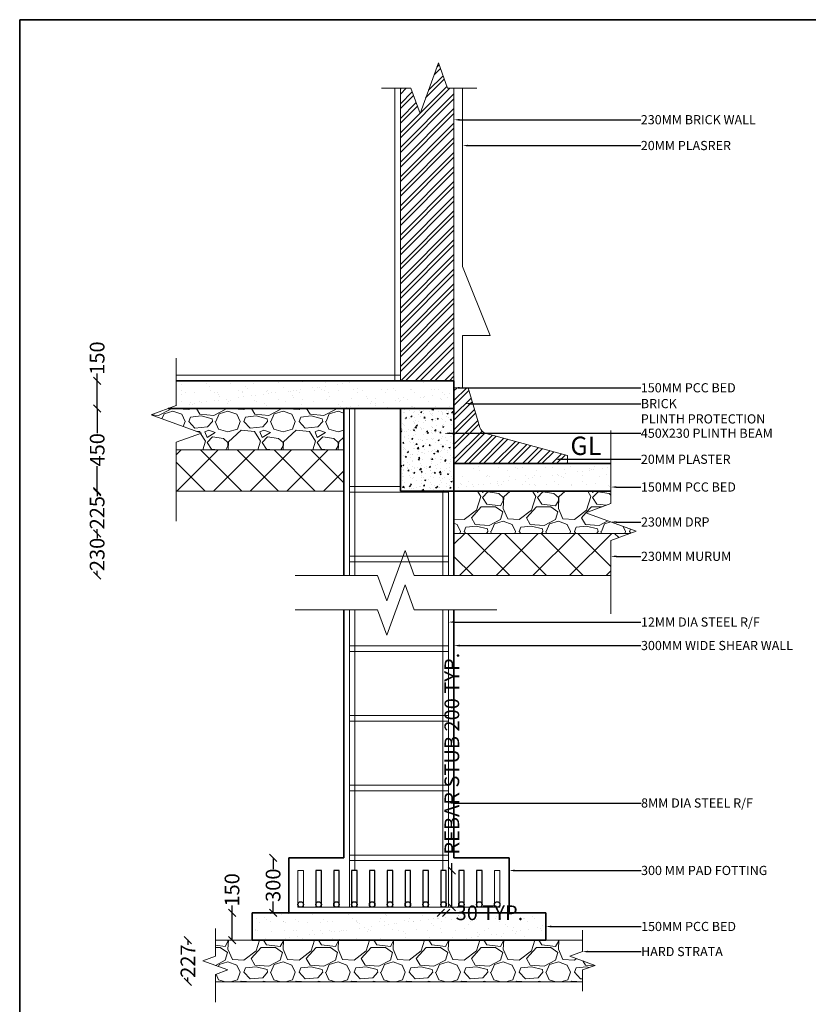
# Model space of a CAD drawing. Units: millimetres. Extents: x -6233 to 6805, y -5269 to 4890.
# Tile 2 of 4: x -6233 to -1936, y -472 to 4890. Entities that reach past the tile are written whole.
import ezdxf
from ezdxf import colors
from ezdxf.entities.mleader import LeaderData, LeaderLine
from ezdxf.math import Vec2, Vec3

# ---------------------------------------------------------------- set-up
doc = ezdxf.new("R2010")
doc.units = ezdxf.units.MM
doc.header["$MEASUREMENT"] = 0
for name, color, linetype, lineweight in [('S-ANNO-DIMS', 2, 'Continuous', 18), ('S-ANNO-TEXT', 3, 'Continuous', 18), ('S-ANNO-TTLB', 7, 'Continuous', 35), ('S-CONC', 7, 'Continuous', 35), ('S-FNDN', 8, 'Continuous', 18), ('S-PATT', 252, 'Continuous', 13), ('S-REIN', 1, 'Continuous', 25)]:
    doc.layers.add(name, color=color, linetype=linetype, lineweight=lineweight)
doc.styles.get("Standard").update_dxf_attribs({"font": 'arial.ttf'})
doc.dimstyles.get("Standard").update_dxf_attribs({"dimtxt": 80, "dimasz": 40, "dimexe": 0.18, "dimexo": 0.0625, "dimgap": 0.09, "dimtad": 0, "dimdec": 0, "dimzin": 0, "dimdsep": 46, "dimtxsty": 'Standard', "dimblk": 'OBLIQUE', "dimcen": 0.09, "dimadec": 0, "dimazin": 0, "dimtfac": 1, "dimtdec": 0, "dimtofl": 0, "dimtmove": 0, "dimatfit": 3, "dimfxl": 1, "dimfxlon": 1, "dimtolj": 1, "dimtzin": 0, "dimarcsym": 0})

# ---------------------------------------------------------------- blocks, each defined once
blk = doc.blocks.new('_Oblique')
at = {"color": 0, "linetype": 'ByBlock', "lineweight": -2}
blk.add_line((-0.5, -0.5), (0.5, 0.5), dxfattribs=at)
blk = doc.blocks.new('*D2')
at = {"layer": 'DEFPOINTS', "color": 0, "transparency": 16777216}
for p in [(-5316.4, -123.9), (-5166.8, -123.9), (-5166.8, -350.9)]:
    blk.add_point(p, dxfattribs=at)
at = {"layer": 'S-ANNO-DIMS', "color": 0, "lineweight": -2, "transparency": 16777216}
for p, q in [((-5315.4, -123.9), (-5316.6, -123.9)), ((-5316.4, -123.9), (-5316.4, -148.2)), ((-5315.4, -350.9), (-5316.6, -350.9)), ((-5316.4, -350.9), (-5316.4, -326.5))]:
    blk.add_line(p, q, dxfattribs=at)
at = {"layer": 'S-ANNO-DIMS', "color": 0, "lineweight": -2, "transparency": 16777216, "xscale": 40, "yscale": 40, "zscale": 40}
for p, rotation in [((-5316.4, -123.9), 90), ((-5316.4, -350.9), 270)]:
    blk.add_blockref('_Oblique', p, dxfattribs=dict(at, rotation=rotation))
at = {"layer": 'S-ANNO-DIMS', "color": 0, "transparency": 16777216, "insert": (-5316.4, -237.4), "char_height": 80, "attachment_point": 5, "rotation": 90}
blk.add_mtext('\\A1;227', dxfattribs=at)
blk = doc.blocks.new('*D3')
at = {"layer": 'DEFPOINTS', "color": 0, "transparency": 16777216}
for p in [(-5076.2, 26.1), (-4966.8, 26.1), (-4966.8, -123.9)]:
    blk.add_point(p, dxfattribs=at)
at = {"layer": 'S-ANNO-DIMS', "color": 0, "lineweight": -2, "transparency": 16777216}
for p, q in [((-5076.2, 26.1), (-5076.2, 66.1)), ((-5075.2, 26.1), (-5076.4, 26.1)), ((-5076.2, -123.9), (-5076.2, 26.1)), ((-5075.2, -123.9), (-5076.4, -123.9))]:
    blk.add_line(p, q, dxfattribs=at)
at = {"layer": 'S-ANNO-DIMS', "color": 0, "lineweight": -2, "transparency": 16777216, "xscale": 40, "yscale": 40, "zscale": 40}
for p, rotation in [((-5076.2, 26.1), 90), ((-5076.2, -123.9), 270)]:
    blk.add_blockref('_Oblique', p, dxfattribs=dict(at, rotation=rotation))
at = {"layer": 'S-ANNO-DIMS', "color": 0, "transparency": 16777216, "insert": (-5076.2, 150.7), "char_height": 80, "attachment_point": 5, "rotation": 90}
blk.add_mtext('\\A1;150', dxfattribs=at)
blk = doc.blocks.new('*D4')
at = {"layer": 'DEFPOINTS', "color": 0, "transparency": 16777216}
for p in [(-4852.4, 326.1), (-4766.8, 326.1), (-4766.8, 26.1)]:
    blk.add_point(p, dxfattribs=at)
at = {"layer": 'S-ANNO-DIMS', "color": 0, "lineweight": -2, "transparency": 16777216}
for p, q in [((-4851.4, 326.1), (-4852.6, 326.1)), ((-4852.4, 326.1), (-4852.4, 264.4)), ((-4852.4, 26.1), (-4852.4, 87.8)), ((-4851.4, 26.1), (-4852.6, 26.1))]:
    blk.add_line(p, q, dxfattribs=at)
at = {"layer": 'S-ANNO-DIMS', "color": 0, "lineweight": -2, "transparency": 16777216, "xscale": 40, "yscale": 40, "zscale": 40}
for p, rotation in [((-4852.4, 326.1), 90), ((-4852.4, 26.1), 270)]:
    blk.add_blockref('_Oblique', p, dxfattribs=dict(at, rotation=rotation))
at = {"layer": 'S-ANNO-DIMS', "color": 0, "transparency": 16777216, "insert": (-4852.4, 176.1), "char_height": 80, "attachment_point": 5, "rotation": 90}
blk.add_mtext('\\A1;300', dxfattribs=at)
blk = doc.blocks.new('*D5')
at = {"layer": 'DEFPOINTS', "color": 0, "transparency": 16777216}
for p in [(-5810.9, 2092.6), (-3866.8, 2092.6), (-3858.6, 1862.6)]:
    blk.add_point(p, dxfattribs=at)
at = {"layer": 'S-ANNO-DIMS', "color": 0, "lineweight": -2, "transparency": 16777216}
for p, q in [((-5809.9, 2092.6), (-5811.1, 2092.6)), ((-5810.9, 2092.6), (-5810.9, 2066.7)), ((-5810.9, 1862.6), (-5810.9, 1888.6)), ((-5809.9, 1862.6), (-5811.1, 1862.6))]:
    blk.add_line(p, q, dxfattribs=at)
at = {"layer": 'S-ANNO-DIMS', "color": 0, "lineweight": -2, "transparency": 16777216, "xscale": 40, "yscale": 40, "zscale": 40}
for p, rotation in [((-5810.9, 2092.6), 90), ((-5810.9, 1862.6), 270)]:
    blk.add_blockref('_Oblique', p, dxfattribs=dict(at, rotation=rotation))
at = {"layer": 'S-ANNO-DIMS', "color": 0, "transparency": 16777216, "insert": (-5810.9, 1977.6), "char_height": 80, "attachment_point": 5, "rotation": 90}
blk.add_mtext('\\A1;230', dxfattribs=at)
blk = doc.blocks.new('*D6')
at = {"layer": 'DEFPOINTS', "color": 0, "transparency": 16777216}
for p in [(-5811.1, 2317.5), (-3866.8, 2317.5), (-3866.8, 2092.6)]:
    blk.add_point(p, dxfattribs=at)
at = {"layer": 'S-ANNO-DIMS', "color": 0, "lineweight": -2, "transparency": 16777216}
for p, q in [((-5810.1, 2317.5), (-5811.3, 2317.5)), ((-5811.1, 2317.5), (-5811.1, 2294.5)), ((-5810.1, 2092.6), (-5811.3, 2092.6)), ((-5811.1, 2092.6), (-5811.1, 2115.6))]:
    blk.add_line(p, q, dxfattribs=at)
at = {"layer": 'S-ANNO-DIMS', "color": 0, "lineweight": -2, "transparency": 16777216, "xscale": 40, "yscale": 40, "zscale": 40}
for p, rotation in [((-5811.1, 2317.5), 90), ((-5811.1, 2092.6), 270)]:
    blk.add_blockref('_Oblique', p, dxfattribs=dict(at, rotation=rotation))
at = {"layer": 'S-ANNO-DIMS', "color": 0, "transparency": 16777216, "insert": (-5811.1, 2205), "char_height": 80, "attachment_point": 5, "rotation": 90}
blk.add_mtext('\\A1;225', dxfattribs=at)
blk = doc.blocks.new('*D8')
at = {"layer": 'DEFPOINTS', "color": 0, "transparency": 16777216}
for p in [(-5810.7, 2772.6), (-5380, 2772.6), (-5380, 2322.6)]:
    blk.add_point(p, dxfattribs=at)
at = {"layer": 'S-ANNO-DIMS', "color": 0, "lineweight": -2, "transparency": 16777216}
for p, q in [((-5809.7, 2772.6), (-5810.9, 2772.6)), ((-5810.7, 2772.6), (-5810.7, 2637.6)), ((-5810.7, 2322.6), (-5810.7, 2457.7)), ((-5809.7, 2322.6), (-5810.9, 2322.6))]:
    blk.add_line(p, q, dxfattribs=at)
at = {"layer": 'S-ANNO-DIMS', "color": 0, "lineweight": -2, "transparency": 16777216, "xscale": 40, "yscale": 40, "zscale": 40}
for p, rotation in [((-5810.7, 2772.6), 90), ((-5810.7, 2322.6), 270)]:
    blk.add_blockref('_Oblique', p, dxfattribs=dict(at, rotation=rotation))
at = {"layer": 'S-ANNO-DIMS', "color": 0, "transparency": 16777216, "insert": (-5810.7, 2547.6), "char_height": 80, "attachment_point": 5, "rotation": 90}
blk.add_mtext('\\A1;450', dxfattribs=at)
blk = doc.blocks.new('*D9')
at = {"layer": 'DEFPOINTS', "color": 0, "transparency": 16777216}
for p in [(-5810.9, 2922.6), (-5380, 2922.6), (-5423.9, 2772.6)]:
    blk.add_point(p, dxfattribs=at)
at = {"layer": 'S-ANNO-DIMS', "color": 0, "lineweight": -2, "transparency": 16777216}
for p, q in [((-5810.9, 2922.6), (-5810.9, 2962.6)), ((-5809.9, 2922.6), (-5811.1, 2922.6)), ((-5810.9, 2772.6), (-5810.9, 2922.6)), ((-5809.9, 2772.6), (-5811.1, 2772.6))]:
    blk.add_line(p, q, dxfattribs=at)
at = {"layer": 'S-ANNO-DIMS', "color": 0, "lineweight": -2, "transparency": 16777216, "xscale": 40, "yscale": 40, "zscale": 40}
for p, rotation in [((-5810.9, 2922.6), 90), ((-5810.9, 2772.6), 270)]:
    blk.add_blockref('_Oblique', p, dxfattribs=dict(at, rotation=rotation))
at = {"layer": 'S-ANNO-DIMS', "color": 0, "transparency": 16777216, "insert": (-5810.9, 3047.2), "char_height": 80, "attachment_point": 5, "rotation": 90}
blk.add_mtext('\\A1;150', dxfattribs=at)
blk = doc.blocks.new('REBAR-STUB-RAFT')
for p, q in [((0, 200), (0, 50)), ((30, 200), (0, 200)), ((30, 0), (30, 200)), ((0, 50), (0, 0))]:
    blk.add_line(p, q)
blk = doc.blocks.new('*D28')
at = {"layer": 'DEFPOINTS', "color": 0, "transparency": 16777216}
for p in [(-3908.6, 256.1), (-3878.6, 256.1), (-3908.6, 56.1)]:
    blk.add_point(p, dxfattribs=at)
at = {"layer": 'S-ANNO-DIMS', "color": 0, "lineweight": -2, "transparency": 16777216}
for p, q in [((-3878.6, 256.1), (-3878.6, 296.1)), ((-3879.6, 256.1), (-3878.4, 256.1)), ((-3878.6, 56.1), (-3878.6, 256.1)), ((-3879.6, 56.1), (-3878.4, 56.1))]:
    blk.add_line(p, q, dxfattribs=at)
at = {"layer": 'S-ANNO-DIMS', "color": 0, "lineweight": -2, "transparency": 16777216, "xscale": 40, "yscale": 40, "zscale": 40}
for p, rotation in [((-3878.6, 256.1), 90), ((-3878.6, 56.1), 270)]:
    blk.add_blockref('_Oblique', p, dxfattribs=dict(at, rotation=rotation))
at = {"layer": 'S-ANNO-DIMS', "color": 0, "transparency": 16777216, "insert": (-3878.6, 892.5), "char_height": 80, "attachment_point": 5, "rotation": 90}
blk.add_mtext('\\A1;REBAR STUB 200 TYP.', dxfattribs=at)
blk = doc.blocks.new('*D29')
at = {"layer": 'DEFPOINTS', "color": 0, "transparency": 16777216}
for p in [(-3938.6, 56.1), (-3908.6, 56.1), (-3908.6, 26.1)]:
    blk.add_point(p, dxfattribs=at)
at = {"layer": 'S-ANNO-DIMS', "color": 0, "lineweight": -2, "transparency": 16777216}
for p, q in [((-3938.6, 27.1), (-3938.6, 26)), ((-3938.6, 26.1), (-3908.6, 26.1)), ((-3908.6, 27.1), (-3908.6, 26)), ((-3908.6, 26.1), (-3868.6, 26.1))]:
    blk.add_line(p, q, dxfattribs=at)
at = {"layer": 'S-ANNO-DIMS', "color": 0, "lineweight": -2, "transparency": 16777216, "xscale": 40, "yscale": 40, "zscale": 40, "rotation": 180}
blk.add_blockref('_Oblique', (-3938.6, 26.1), dxfattribs=at)
at = {"layer": 'S-ANNO-DIMS', "color": 0, "lineweight": -2, "transparency": 16777216, "xscale": 40, "yscale": 40, "zscale": 40}
blk.add_blockref('_Oblique', (-3908.6, 26.1), dxfattribs=at)
at = {"layer": 'S-ANNO-DIMS', "color": 0, "transparency": 16777216, "insert": (-3673.8, 26.1), "char_height": 80, "attachment_point": 5}
blk.add_mtext('\\A1;30 TYP.', dxfattribs=at)

msp = doc.modelspace()

# ---------------------------------------------------------------- hatches: boundary and pattern name
at = {"layer": 'S-PATT'}
h = msp.add_hatch(dxfattribs=at)
h.set_pattern_fill('ANSI32', color=256, scale=150)
h.paths.add_polyline_path([(-4158.9, 2922.6), (-3866.8, 2922.6), (-3866.8, 4517.1), (-3901.9, 4517.1), (-3951.9, 4654.5), (-4051.9, 4379.8), (-4101.9, 4517.1), (-4158.9, 4517.1)])
h.paths.add_polyline_path([(-3790.4, 2885.1), (-3866.8, 2885.1), (-3866.8, 2472.6), (-3248.6, 2472.6), (-3248.6, 2517.5), (-3690.8, 2636.1, -0.259704), (-3725.7, 2670)])
h = msp.add_hatch(dxfattribs=at)
h.set_pattern_fill('AR-SAND', color=256, scale=50)
h.paths.add_polyline_path([(-3866.8, 2772.6), (-3866.8, 2922.6), (-5380, 2922.6), (-5380, 2788.6), (-5423.9, 2772.6)])
h.paths.add_polyline_path([(-3011.9, 2322.6), (-3011.9, 2472.6), (-3866.8, 2472.6), (-3866.8, 2322.6)])
h.paths.add_polyline_path([(-4966.8, 26.1), (-4966.8, -123.9), (-3366.8, -123.9), (-3366.8, 26.1), (-3566.8, 26.1)])
h = msp.add_hatch(dxfattribs=at)
h.set_pattern_fill('GRAVEL', color=256, scale=300)
h.paths.add_polyline_path([(-5423.9, 2772.6), (-5517.4, 2738.6), (-5242.6, 2638.6), (-5380, 2588.6), (-5380, 2547.6), (-4466.8, 2547.6), (-4466.8, 2772.6)])
h.paths.add_polyline_path([(-3866.8, 2322.6), (-3866.8, 2092.6), (-2906.5, 2092.6), (-2874.6, 2104.3), (-3149.3, 2204.3), (-3011.9, 2254.3), (-3011.9, 2322.6)])
h.paths.add_polyline_path([(-3166.8, -350.9), (-3166.8, -285.5), (-3098.1, -260.5), (-3235.5, -210.5), (-3166.8, -185.5), (-3166.8, -123.9), (-3366.8, -123.9), (-4966.8, -123.9), (-5166.8, -123.9), (-5166.8, -210.2), (-5235.5, -235.2), (-5098.1, -285.2), (-5166.8, -310.2), (-5166.8, -350.9)])
h = msp.add_hatch(dxfattribs=at)
h.set_pattern_fill('AR-CONC', color=256, scale=10)
h.paths.add_polyline_path([(-4158.9, 2322.6), (-3866.8, 2322.6), (-3866.8, 2772.6), (-4158.9, 2772.6)])
h = msp.add_hatch(dxfattribs=at)
h.set_pattern_fill('¶À¿×²ÄÁÏ', color=256, scale=50)
h.set_pattern_definition([(45, (100, 0), (-100, 100), []), (135, (100, 0), (-100, -100), [])])
h.paths.add_polyline_path([(-4466.8, 2322.6), (-4466.8, 2547.6), (-5380, 2547.6), (-5380, 2322.6)])
h.paths.add_polyline_path([(-3866.8, 2092.6), (-3866.8, 1862.6), (-3011.9, 1862.6), (-3011.9, 2054.3), (-2906.5, 2092.6)])

# ---------------------------------------------------------------- linework, layer by layer
at = {"layer": 'S-ANNO-TTLB'}
msp.add_lwpolyline([(-6232.9, 4890.2), (2600.5, 4890.2), (2600.5, -1330.2), (-6232.9, -1330.2)], close=True, dxfattribs=at)
at = {"layer": 'S-CONC'}
for p, q in [((-3866.8, 2922.6), (-5380, 2922.6)), ((-3866.8, 2922.6), (-3866.8, 1862.6)), ((-3866.8, 2772.6), (-5423.9, 2772.6)), ((-4466.8, 2772.6), (-4466.8, 1862.6)), ((-4158.9, 2322.6), (-4158.9, 2772.6)), ((-3866.8, 2472.6), (-3011.9, 2472.6)), ((-3866.8, 2322.6), (-4158.9, 2322.6)), ((-3866.8, 2322.6), (-3011.9, 2322.6)), ((-4466.8, 326.1), (-4466.8, 1675.2)), ((-3866.8, 326.1), (-3866.8, 1675.2)), ((-4766.8, 26.1), (-4766.8, 326.1)), ((-4766.8, 326.1), (-4466.8, 326.1)), ((-3566.8, 326.1), (-3866.8, 326.1)), ((-3566.8, 26.1), (-3566.8, 326.1)), ((-4966.8, 26.1), (-3366.8, 26.1)), ((-4966.8, -123.9), (-4966.8, 26.1)), ((-4966.8, 26.1), (-4766.8, 26.1)), ((-3366.8, -123.9), (-3366.8, 26.1)), ((-3366.8, -123.9), (-4966.8, -123.9))]:
    msp.add_line(p, q, dxfattribs=at)
at = {"layer": 'S-FNDN'}
for p, q in [((-4188.9, 2922.6), (-4188.9, 4517.1)), ((-4158.9, 2922.6), (-4158.9, 4517.1)), ((-3866.8, 4517.1), (-3866.8, 2922.6)), ((-3819.8, 4517.1), (-3819.8, 3546.1)), ((-3819.8, 3546.1), (-3670.5, 3169.4)), ((-3670.5, 3169.4), (-3819.8, 3169.4)), ((-3819.8, 3169.4), (-3819.8, 2887.3)), ((-4158.9, 2954.4), (-5380, 2954.4)), ((-3866.8, 2885.1), (-3790.4, 2885.1)), ((-3790.4, 2885.1), (-3725.7, 2670)), ((-4436.8, 1862.6), (-4436.8, 2772.6)), ((-4406.8, 1862.6), (-4406.8, 2772.6)), ((-3690.8, 2636.1), (-3248.6, 2517.5)), ((-4466.8, 2547.6), (-5380, 2547.6)), ((-3248.6, 2517.5), (-3248.6, 2472.6)), ((-4466.8, 2322.6), (-5380, 2322.6)), ((-4436.8, 2347.5), (-4158.9, 2347.5)), ((-4436.8, 2317.5), (-3896.8, 2317.5)), ((-3926.8, 1862.6), (-3926.8, 2322.6)), ((-3896.8, 1862.6), (-3896.8, 2322.6)), ((-3866.8, 2092.6), (-2906.5, 2092.6)), ((-4436.8, 1967.6), (-3896.8, 1967.6)), ((-4436.8, 1937.6), (-3896.8, 1937.6)), ((-3866.8, 1862.6), (-3011.9, 1862.6)), ((-4436.8, 56.1), (-4436.8, 1675.2)), ((-4406.8, 256.1), (-4406.8, 1675.2)), ((-3926.8, 256.1), (-3926.8, 1675.2)), ((-3896.8, 56.1), (-3896.8, 1675.2)), ((-4436.8, 1479.8), (-3896.8, 1479.8)), ((-4436.8, 1449.8), (-3896.8, 1449.8)), ((-4436.8, 1100), (-3896.8, 1100)), ((-4436.8, 1070), (-3896.8, 1070)), ((-4436.8, 720.2), (-3896.8, 720.2)), ((-4436.8, 690.2), (-3896.8, 690.2)), ((-4766.8, 326.1), (-4466.8, 326.1)), ((-4436.8, 340.3), (-3896.8, 340.3)), ((-3866.8, 326.1), (-3566.8, 326.1)), ((-4436.8, 310.3), (-3896.8, 310.3)), ((-4716.8, 256.1), (-4716.8, 106.1)), ((-4686.8, 256.1), (-4716.8, 256.1)), ((-4686.8, 56.1), (-4686.8, 256.1)), ((-3646.8, 256.1), (-3646.8, 106.1)), ((-3616.8, 256.1), (-3646.8, 256.1)), ((-3616.8, 56.1), (-3616.8, 256.1)), ((-4716.8, 106.1), (-4716.8, 56.1)), ((-4716.8, 56.1), (-3616.8, 56.1)), ((-4716.8, 56.1), (-4686.8, 56.1)), ((-3646.8, 106.1), (-3646.8, 56.1)), ((-3366.8, 26.1), (-3566.8, 26.1)), ((-5166.8, -123.9), (-4966.8, -123.9)), ((-3366.8, -123.9), (-3166.8, -123.9)), ((-5166.8, -350.9), (-3166.8, -350.9))]:
    msp.add_line(p, q, dxfattribs=at)
for points in [[(-4261.5, 4517.1), (-4101.9, 4517.1), (-4051.9, 4379.8), (-3951.9, 4654.5), (-3901.9, 4517.1), (-3742.2, 4517.1)], [(-5380, 3046), (-5380, 2788.6), (-5517.4, 2738.6), (-5242.6, 2638.6), (-5380, 2588.6), (-5380, 2159.3)], [(-3011.9, 2653.5), (-3011.9, 2254.3), (-3149.3, 2204.3), (-2874.6, 2104.3), (-3011.9, 2054.3), (-3011.9, 1655)], [(-4732.7, 1862.6), (-4283.3, 1862.6), (-4233.3, 1725.3), (-4133.3, 2000), (-4083.3, 1862.6), (-3633.9, 1862.6)], [(-4732.5, 1675.2), (-4283.3, 1675.2), (-4233.3, 1537.8), (-4133.3, 1812.6), (-4083.3, 1675.2), (-3634, 1675.2)], [(-5166.8, -461.4), (-5166.8, -310.2), (-5098.1, -285.2), (-5235.5, -235.2), (-5166.8, -210.2), (-5166.8, -58.9)], [(-3166.8, -401.5), (-3166.8, -285.5), (-3098.1, -260.5), (-3235.5, -210.5), (-3166.8, -185.5), (-3166.8, -69.5)]]:
    msp.add_lwpolyline(points, dxfattribs=at)
msp.add_arc((-3677.8, 2684.4), 50, 196.7477, 254.9811, dxfattribs=at)
at = {"layer": 'S-REIN'}
for centre in [(-4701.8, 71.1), (-4604.5, 71.1), (-4507.2, 71.1), (-4410, 71.1), (-4312.7, 71.1), (-4215.4, 71.1), (-4118.2, 71.1), (-4020.9, 71.1), (-3923.6, 71.1), (-3826.3, 71.1), (-3729.1, 71.1), (-3631.8, 71.1)]:
    msp.add_circle(centre, 15, dxfattribs=at)

# ---------------------------------------------------------------- block references
for p in [(-4619.5, 56.1), (-4522.2, 56.1), (-4425, 56.1), (-4327.7, 56.1), (-4230.4, 56.1), (-4133.2, 56.1), (-4035.9, 56.1), (-3938.6, 56.1), (-3841.3, 56.1), (-3744.1, 56.1)]:
    msp.add_blockref('REBAR-STUB-RAFT', p, dxfattribs=at)

# ---------------------------------------------------------------- texts
at = {"layer": 'S-ANNO-TEXT', "insert": (-3232.5, 2619.5), "char_height": 100, "attachment_point": 1}
msp.add_mtext_dynamic_manual_height_columns('GL', width=751.493, gutter_width=1, heights=[0], dxfattribs=at)

# ---------------------------------------------------------------- dimensions: what is measured, and where the dimension line sits
at = {"layer": 'S-ANNO-DIMS'}
for base, p1, p2, picture, middle in [((-5810.9, 2922.6), (-5423.9, 2772.6), (-5380, 2922.6), '*D9', (-5810.9, 3047.2)), ((-5810.7, 2772.6), (-5380, 2322.6), (-5380, 2772.6), '*D8', (-5810.7, 2547.6)), ((-5811.1, 2317.5), (-3866.8, 2092.6), (-3866.8, 2317.5), '*D6', (-5811.1, 2205)), ((-5810.9, 2092.6), (-3858.6, 1862.6), (-3866.8, 2092.6), '*D5', (-5810.9, 1977.6)), ((-4852.4, 326.1), (-4766.8, 26.1), (-4766.8, 326.1), '*D4', (-4852.4, 176.1)), ((-5076.2, 26.1), (-4966.8, -123.9), (-4966.8, 26.1), '*D3', (-5076.2, 150.7)), ((-5316.4, -123.9), (-5166.8, -350.9), (-5166.8, -123.9), '*D2', (-5316.4, -237.4))]:
    dim = msp.add_linear_dim(base=base, p1=p1, p2=p2, angle=90, dimstyle='Standard', override={"dimclrd": 0, "dimclre": 0, "dimclrt": 0}, dxfattribs=at)
    dim.commit()
    dim.dimension.update_dxf_attribs({"geometry": picture, "text_midpoint": middle})
dim = msp.add_linear_dim(base=(-3878.6, 256.1), p1=(-3908.6, 56.1), p2=(-3908.6, 256.1), angle=90, text='REBAR STUB <> TYP.', dimstyle='Standard', override={"dimdec": 0, "dimrnd": 0, "dimzin": 0, "dimlunit": 2}, dxfattribs=at)
dim.commit()
dim.dimension.update_dxf_attribs({"geometry": '*D28', "text_midpoint": (-3878.6, 892.5)})
dim = msp.add_linear_dim(base=(-3908.6, 26.1), p1=(-3938.6, 56.1), p2=(-3908.6, 56.1), text='<> TYP.', dimstyle='Standard', override={"dimdec": 0, "dimrnd": 0, "dimzin": 0, "dimlunit": 2}, dxfattribs=at)
dim.commit()
dim.dimension.update_dxf_attribs({"geometry": '*D29', "text_midpoint": (-3673.8, 26.1)})

# ---------------------------------------------------------------- leaders
at = {"layer": 'S-ANNO-TEXT'}
ml = msp.add_multileader_mtext('Standard', dxfattribs=at)
ml.set_content('230MM BRICK WALL', color=256)
ml.set_leader_properties()
ml.build(insert=Vec2(0, 0))
ml.multileader.update_dxf_attribs({"dogleg_length": 0.36, "arrow_head_size": 30})
ctx = ml.context
ctx.base_point, ctx.char_height, ctx.arrow_head_size, ctx.landing_gap_size, ctx.plane_origin = Vec3(-2849.1, 4345.1), 50, 30, 0.09, Vec3(-3866.8, 4345.1)
notes = []
notes.append((ctx, [(0, (1, 1, 0), (-2849.5, 4345.1), (1, 0), 0.36, [(0, [(-3866.8, 4345.1)], 0, [])])]))
ctx.mtext.insert, ctx.mtext.flow_direction = Vec3(-2849, 4370.5), 5
ml = msp.add_multileader_mtext('Standard', dxfattribs=at)
ml.set_content('20MM PLASRER', color=256)
ml.set_leader_properties()
ml.build(insert=Vec2(0, 0))
ml.multileader.update_dxf_attribs({"dogleg_length": 0.36, "arrow_head_size": 30})
ctx = ml.context
ctx.base_point, ctx.char_height, ctx.arrow_head_size, ctx.landing_gap_size, ctx.plane_origin = Vec3(-2849.1, 4204.5), 50, 30, 0.09, Vec3(-3819.8, 4204.5)
notes.append((ctx, [(0, (1, 1, 0), (-2849.5, 4204.5), (1, 0), 0.36, [(0, [(-3819.8, 4204.5)], 0, [])])]))
ctx.mtext.insert, ctx.mtext.flow_direction = Vec3(-2849, 4229.9), 5
ml = msp.add_multileader_mtext('Standard', dxfattribs=at)
ml.set_content('150MM PCC BED', color=256)
ml.set_leader_properties()
ml.build(insert=Vec2(0, 0))
ml.multileader.update_dxf_attribs({"dogleg_length": 0.36, "arrow_head_size": 30})
ctx = ml.context
ctx.base_point, ctx.char_height, ctx.arrow_head_size, ctx.landing_gap_size, ctx.plane_origin = Vec3(-2849.1, 2885.1), 50, 30, 0.09, Vec3(-3866.8, 2885.1)
notes.append((ctx, [(0, (1, 1, 0), (-2849.5, 2885.1), (1, 0), 0.36, [(0, [(-3866.8, 2885.1)], 0, [])])]))
ctx.mtext.insert, ctx.mtext.flow_direction = Vec3(-2849, 2910.5), 5
ml = msp.add_multileader_mtext('Standard', dxfattribs=at)
ml.set_content('BRICK\\PPLINTH PROTECTION', color=256)
ml.set_leader_properties()
ml.build(insert=Vec2(0, 0))
ml.multileader.update_dxf_attribs({"dogleg_length": 0.36, "arrow_head_size": 30})
ctx = ml.context
ctx.base_point, ctx.char_height, ctx.arrow_head_size, ctx.landing_gap_size, ctx.plane_origin = Vec3(-2848.8, 2798.9), 50, 30, 0.09, Vec3(-3807.9, 2798.9)
notes.append((ctx, [(0, (1, 1, 0), (-2849.1, 2798.9), (1, 0), 0.36, [(0, [(-3807.9, 2798.9)], 0, [])])]))
ctx.mtext.insert, ctx.mtext.flow_direction = Vec3(-2848.7, 2824.3), 5
ml = msp.add_multileader_mtext('Standard', dxfattribs=at)
ml.set_content('450X230 PLINTH BEAM', color=256)
ml.set_leader_properties()
ml.build(insert=Vec2(0, 0))
ml.multileader.update_dxf_attribs({"dogleg_length": 0.36, "arrow_head_size": 30})
ctx = ml.context
ctx.base_point, ctx.char_height, ctx.arrow_head_size, ctx.landing_gap_size, ctx.plane_origin = Vec3(-2848.8, 2637.6), 50, 30, 0.09, Vec3(-3920.5, 2637.6)
notes.append((ctx, [(0, (1, 1, 0), (-2849.1, 2637.6), (1, 0), 0.36, [(0, [(-3920.5, 2637.6)], 0, [])])]))
ctx.mtext.insert, ctx.mtext.flow_direction = Vec3(-2848.7, 2663), 5
ml = msp.add_multileader_mtext('Standard', dxfattribs=at)
ml.set_content('20MM PLASTER', color=256)
ml.set_leader_properties()
ml.build(insert=Vec2(0, 0))
ml.multileader.update_dxf_attribs({"dogleg_length": 0.36, "arrow_head_size": 30})
ctx = ml.context
ctx.base_point, ctx.char_height, ctx.arrow_head_size, ctx.landing_gap_size, ctx.plane_origin = Vec3(-2848.8, 2495.8), 50, 30, 0.09, Vec3(-3316.4, 2495.8)
notes.append((ctx, [(0, (1, 1, 0), (-2849.1, 2495.8), (1, 0), 0.36, [(0, [(-3316.4, 2495.8)], 0, [])])]))
ctx.mtext.insert, ctx.mtext.flow_direction = Vec3(-2848.7, 2521.2), 5
ml = msp.add_multileader_mtext('Standard', dxfattribs=at)
ml.set_content('150MM PCC BED', color=256)
ml.set_leader_properties()
ml.build(insert=Vec2(0, 0))
ml.multileader.update_dxf_attribs({"dogleg_length": 0.36, "arrow_head_size": 30})
ctx = ml.context
ctx.base_point, ctx.char_height, ctx.arrow_head_size, ctx.landing_gap_size, ctx.plane_origin = Vec3(-2848.4, 2344.7), 50, 30, 0.09, Vec3(-3011.9, 2344.7)
notes.append((ctx, [(0, (1, 1, 0), (-2848.8, 2344.7), (1, 0), 0.36, [(0, [(-3011.9, 2344.7)], 0, [])])]))
ctx.mtext.insert, ctx.mtext.flow_direction = Vec3(-2848.3, 2370.1), 5
ml = msp.add_multileader_mtext('Standard', dxfattribs=at)
ml.set_content('230MM DRP', color=256)
ml.set_leader_properties()
ml.build(insert=Vec2(0, 0))
ml.multileader.update_dxf_attribs({"dogleg_length": 0.36, "arrow_head_size": 30})
ctx = ml.context
ctx.base_point, ctx.char_height, ctx.arrow_head_size, ctx.landing_gap_size, ctx.plane_origin = Vec3(-2848.1, 2154.3), 50, 30, 0.09, Vec3(-3011.9, 2154.3)
notes.append((ctx, [(0, (1, 1, 0), (-2848.4, 2154.3), (1, 0), 0.36, [(0, [(-3011.9, 2154.3)], 0, [])])]))
ctx.mtext.insert, ctx.mtext.flow_direction = Vec3(-2848, 2179.7), 5
ml = msp.add_multileader_mtext('Standard', dxfattribs=at)
ml.set_content('230MM MURUM', color=256)
ml.set_leader_properties()
ml.build(insert=Vec2(0, 0))
ml.multileader.update_dxf_attribs({"dogleg_length": 0.36, "arrow_head_size": 30})
ctx = ml.context
ctx.base_point, ctx.char_height, ctx.arrow_head_size, ctx.landing_gap_size, ctx.plane_origin = Vec3(-2848.1, 1967.3), 50, 30, 0.09, Vec3(-3011.9, 1967.3)
notes.append((ctx, [(0, (1, 1, 0), (-2848.4, 1967.3), (1, 0), 0.36, [(0, [(-3011.9, 1967.3)], 0, [])])]))
ctx.mtext.insert, ctx.mtext.flow_direction = Vec3(-2848, 1992.7), 5
ml = msp.add_multileader_mtext('Standard', dxfattribs=at)
ml.set_content('12MM DIA STEEL R/F', color=256)
ml.set_leader_properties()
ml.build(insert=Vec2(0, 0))
ml.multileader.update_dxf_attribs({"dogleg_length": 0.36, "arrow_head_size": 30})
ctx = ml.context
ctx.base_point, ctx.char_height, ctx.arrow_head_size, ctx.landing_gap_size, ctx.plane_origin = Vec3(-2848.1, 1609.2), 50, 30, 0.09, Vec3(-3896.8, 1609.2)
notes.append((ctx, [(0, (1, 1, 0), (-2848.4, 1609.2), (1, 0), 0.36, [(0, [(-3896.8, 1609.2)], 0, [])])]))
ctx.mtext.insert, ctx.mtext.flow_direction = Vec3(-2848, 1634.6), 5
ml = msp.add_multileader_mtext('Standard', dxfattribs=at)
ml.set_content('300MM WIDE SHEAR WALL', color=256)
ml.set_leader_properties()
ml.build(insert=Vec2(0, 0))
ml.multileader.update_dxf_attribs({"dogleg_length": 0.36, "arrow_head_size": 30})
ctx = ml.context
ctx.base_point, ctx.char_height, ctx.arrow_head_size, ctx.landing_gap_size, ctx.plane_origin = Vec3(-2848.1, 1481.2), 50, 30, 0.09, Vec3(-3866.8, 1481.2)
notes.append((ctx, [(0, (1, 1, 0), (-2848.4, 1481.2), (1, 0), 0.36, [(0, [(-3866.8, 1481.2)], 0, [])])]))
ctx.mtext.insert, ctx.mtext.flow_direction = Vec3(-2848, 1506.7), 5
ml = msp.add_multileader_mtext('Standard', dxfattribs=at)
ml.set_content('8MM DIA STEEL R/F', color=256)
ml.set_leader_properties()
ml.build(insert=Vec2(0, 0))
ml.multileader.update_dxf_attribs({"dogleg_length": 0.36, "arrow_head_size": 30})
ctx = ml.context
ctx.base_point, ctx.char_height, ctx.arrow_head_size, ctx.landing_gap_size, ctx.plane_origin = Vec3(-2847.6, 623.6), 50, 30, 0.09, Vec3(-3896.8, 623.6)
notes.append((ctx, [(0, (1, 1, 0), (-2848, 623.6), (1, 0), 0.36, [(0, [(-3896.8, 623.6)], 0, [])])]))
ctx.mtext.insert, ctx.mtext.flow_direction = Vec3(-2847.5, 649.1), 5
ml = msp.add_multileader_mtext('Standard', dxfattribs=at)
ml.set_content('300 MM PAD FOTTING', color=256)
ml.set_leader_properties()
ml.build(insert=Vec2(0, 0))
ml.multileader.update_dxf_attribs({"dogleg_length": 0.36, "arrow_head_size": 30})
ctx = ml.context
ctx.base_point, ctx.char_height, ctx.arrow_head_size, ctx.landing_gap_size, ctx.plane_origin = Vec3(-2847.6, 256.1), 50, 30, 0.09, Vec3(-3566.8, 256.1)
notes.append((ctx, [(0, (1, 1, 0), (-2848, 256.1), (1, 0), 0.36, [(0, [(-3566.8, 256.1)], 0, [])])]))
ctx.mtext.insert, ctx.mtext.flow_direction = Vec3(-2847.5, 281.6), 5
ml = msp.add_multileader_mtext('Standard', dxfattribs=at)
ml.set_content('150MM PCC BED', color=256)
ml.set_leader_properties()
ml.build(insert=Vec2(0, 0))
ml.multileader.update_dxf_attribs({"dogleg_length": 0.36, "arrow_head_size": 30})
ctx = ml.context
ctx.base_point, ctx.char_height, ctx.arrow_head_size, ctx.landing_gap_size, ctx.plane_origin = Vec3(-2847.6, -48.9), 50, 30, 0.09, Vec3(-3366.8, -48.9)
notes.append((ctx, [(0, (1, 1, 0), (-2848, -48.9), (1, 0), 0.36, [(0, [(-3366.8, -48.9)], 0, [])])]))
ctx.mtext.insert, ctx.mtext.flow_direction = Vec3(-2847.5, -23.4), 5
ml = msp.add_multileader_mtext('Standard', dxfattribs=at)
ml.set_content('HARD STRATA', color=256)
ml.set_leader_properties()
ml.build(insert=Vec2(0, 0))
ml.multileader.update_dxf_attribs({"dogleg_length": 0.36, "arrow_head_size": 30})
ctx = ml.context
ctx.base_point, ctx.char_height, ctx.arrow_head_size, ctx.landing_gap_size, ctx.plane_origin = Vec3(-2847.6, -185.5), 50, 30, 0.09, Vec3(-3166.8, -185.5)
notes.append((ctx, [(0, (1, 1, 0), (-2848, -185.5), (1, 0), 0.36, [(0, [(-3166.8, -185.5)], 0, [])])]))
ctx.mtext.insert, ctx.mtext.flow_direction = Vec3(-2847.5, -160.1), 5
for ctx, leaders in notes:
    for number, flags, end, landing, length, lines in leaders:
        leader = LeaderData()
        leader.index, (leader.has_last_leader_line, leader.has_dogleg_vector, leader.attachment_direction) = number, flags
        leader.last_leader_point, leader.dogleg_vector, leader.dogleg_length = Vec3(end), Vec3(landing), length
        for number, points, colour, breaks in lines:
            line = LeaderLine()
            line.index, line.vertices, line.color, line.breaks = number, Vec3.list(points), colors.encode_raw_color(colour), breaks
            leader.lines.append(line)
        ctx.leaders.append(leader)

doc.saveas('drawing.dxf')
